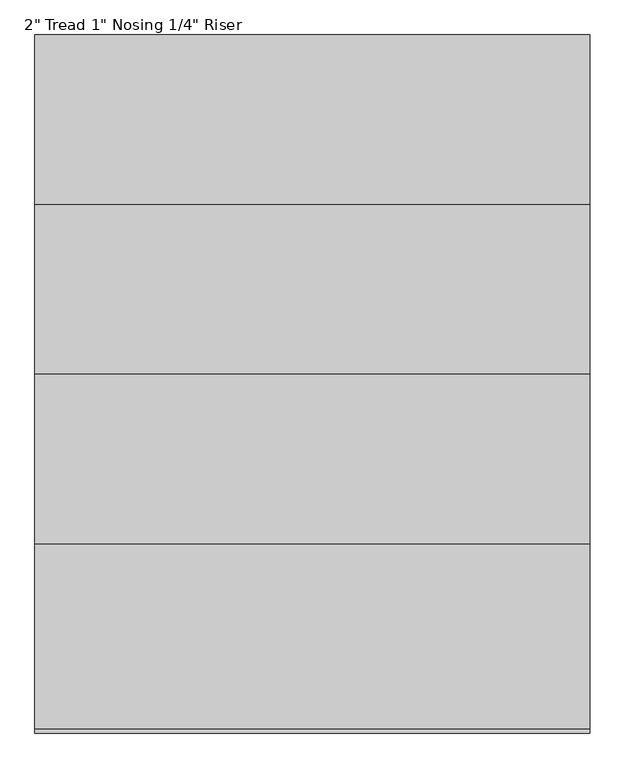
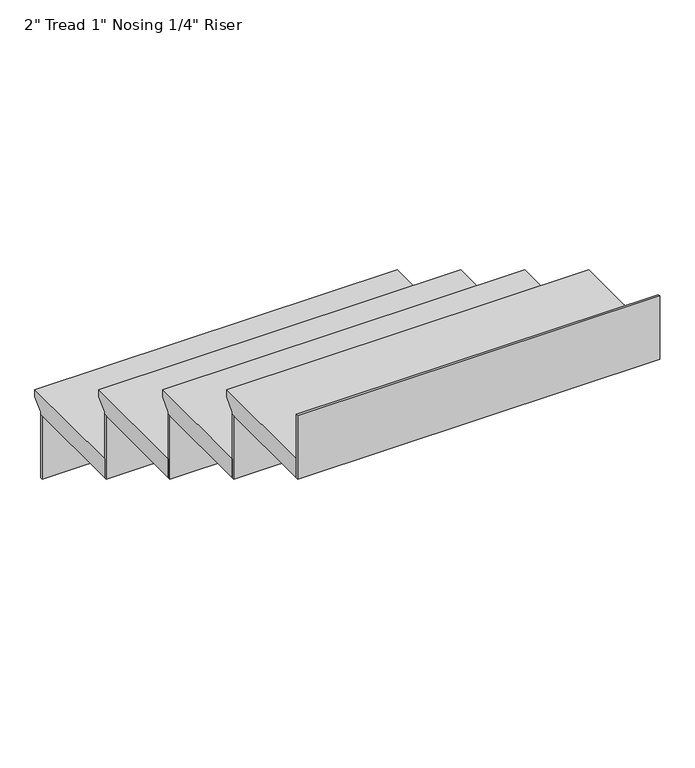
"""IFC4 building model written with IfcOpenShell, lengths in millimetres: stair flight geometry."""

from ifc_helpers import new_model, si_unit, frame, origin, place, context, project, spatial, polyline, outline, extrude, source, transform, mapped, element, save


def stair_flight_57f2103d(model_context):
    return source(origin(), model_context, "Body", "SweptSolid", [
        extrude(outline(polyline([(22889.9216096, 51989.2839133), (23194.7216096, 51989.2839133), (23194.7216096, 51970.2339133), (23169.3216096, 51944.8339133), (23169.3216096, 51938.4839133), (22889.9216096, 51938.4839133), (22889.9216096, 51989.2839133)])), frame((-2398.2415084, 0.0, 0.0), z_axis=(1.0, 0.0, 0.0), x_axis=(0.0, 1.0, 0.0)), (0.0, 0.0, 1.0), 914.4),
        extrude(outline(polyline([(-2398.2415084, 23162.9716096), (-2398.2415084, 23169.3216096), (-1483.8415084, 23169.3216096), (-1483.8415084, 23162.9716096), (-2398.2415084, 23162.9716096)])), frame((0.0, 0.0, 51769.1505799), z_axis=(0.0, 0.0, 1.0), x_axis=(1.0, 0.0, 0.0)), (0.0, 0.0, 1.0), 169.3333333),
        extrude(outline(polyline([(-2398.2415084, 22883.5716096), (-2398.2415084, 22889.9216096), (-1483.8415084, 22889.9216096), (-1483.8415084, 22883.5716096), (-2398.2415084, 22883.5716096)])), frame((0.0, 0.0, 51938.4839133), z_axis=(0.0, 0.0, 1.0), x_axis=(1.0, 0.0, 0.0)), (0.0, 0.0, 1.0), 169.3333333),
        extrude(outline(polyline([(22610.5216096, 52158.6172466), (22915.3216096, 52158.6172466), (22915.3216096, 52139.5672466), (22889.9216096, 52114.1672466), (22889.9216096, 52107.8172466), (22610.5216096, 52107.8172466), (22610.5216096, 52158.6172466)])), frame((-2398.2415084, 0.0, 0.0), z_axis=(1.0, 0.0, 0.0), x_axis=(0.0, 1.0, 0.0)), (0.0, 0.0, 1.0), 914.4),
        extrude(outline(polyline([(-2398.2415084, 22604.1716096), (-2398.2415084, 22610.5216096), (-1483.8415084, 22610.5216096), (-1483.8415084, 22604.1716096), (-2398.2415084, 22604.1716096)])), frame((0.0, 0.0, 52107.8172466), z_axis=(0.0, 0.0, 1.0), x_axis=(1.0, 0.0, 0.0)), (0.0, 0.0, 1.0), 169.3333333),
        extrude(outline(polyline([(22331.1216096, 52327.9505799), (22635.9216096, 52327.9505799), (22635.9216096, 52308.9005799), (22610.5216096, 52283.5005799), (22610.5216096, 52277.1505799), (22331.1216096, 52277.1505799), (22331.1216096, 52327.9505799)])), frame((-2398.2415084, 0.0, 0.0), z_axis=(1.0, 0.0, 0.0), x_axis=(0.0, 1.0, 0.0)), (0.0, 0.0, 1.0), 914.4),
        extrude(outline(polyline([(-2398.2415084, 22324.7716096), (-2398.2415084, 22331.1216096), (-1483.8415084, 22331.1216096), (-1483.8415084, 22324.7716096), (-2398.2415084, 22324.7716096)])), frame((0.0, 0.0, 52277.1505799), z_axis=(0.0, 0.0, 1.0), x_axis=(1.0, 0.0, 0.0)), (0.0, 0.0, 1.0), 169.3333333),
        extrude(outline(polyline([(-2398.2415084, 22045.3716096), (-2398.2415084, 22051.7216096), (-1483.8415084, 22051.7216096), (-1483.8415084, 22045.3716096), (-2398.2415084, 22045.3716096)])), frame((0.0, 0.0, 52446.4839133), z_axis=(0.0, 0.0, 1.0), x_axis=(1.0, 0.0, 0.0)), (0.0, 0.0, 1.0), 169.3333333),
        extrude(outline(polyline([(22051.7216096, 52497.2839133), (22356.5216096, 52497.2839133), (22356.5216096, 52478.2339133), (22331.1216096, 52452.8339133), (22331.1216096, 52446.4839133), (22051.7216096, 52446.4839133), (22051.7216096, 52497.2839133)])), frame((-2398.2415084, 0.0, 0.0), z_axis=(1.0, 0.0, 0.0), x_axis=(0.0, 1.0, 0.0)), (0.0, 0.0, 1.0), 914.4),
    ])


if __name__ == "__main__":
    model = new_model("IFC4")
    model_context = context("Model", 3, world=origin())
    ifc_project = project(units=[si_unit("LENGTHUNIT", "METRE", prefix="MILLI")], contexts=[model_context])
    site = spatial("IfcSite", under=ifc_project)
    building = spatial("IfcBuilding", under=site)
    placement = place(None, origin())
    stair_flight_shape = stair_flight_57f2103d(model_context)
    element("IfcStairFlight", 1, ObjectType="2\" Tread 1\" Nosing 1/4\" Riser", at=placement, inside=building, context=model_context, shape_type="MappedRepresentation", body=[
        mapped(stair_flight_shape, transform((0.0, 0.0, 0.0), x_axis=(1.0, 0.0, 0.0), y_axis=(0.0, 1.0, 0.0), z_axis=(0.0, 0.0, 1.0))),
    ])
    save(model, "model.ifc")
